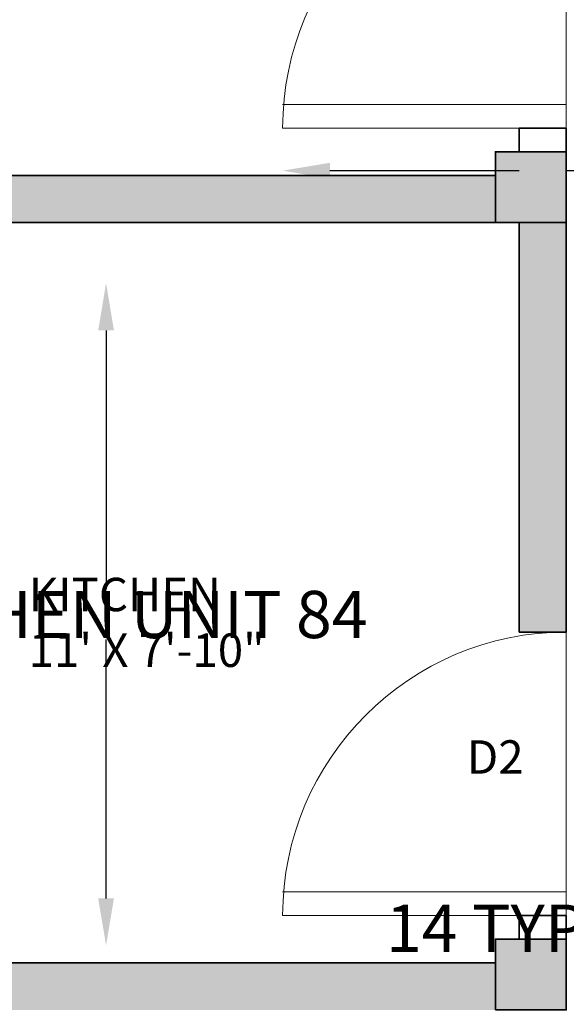
# Model space of a CAD drawing. Units: inches. Extents: x 1994 to 3075, y 3517 to 3950.
# Tile 51 of 58: x 2747 to 2816, y 3656 to 3781. Entities that reach past the tile are written whole.
import ezdxf

# ---------------------------------------------------------------- set-up
doc = ezdxf.new("R2010")
doc.units = ezdxf.units.IN
for name, color, linetype, lineweight in [('A-ANNO-DIMS', 2, 'Continuous', 18), ('A-ANNO-TEXT', 7, 'Continuous', 18), ('A-AREA-IDEN', 7, 'Continuous', 18), ('A-COLS', 7, 'Continuous', 35), ('A-COLS-PATT', 6, 'Continuous', 13), ('A-DOOR', 3, 'Continuous', 18), ('A-WALL', 7, 'Continuous', 35), ('A-WALL-PATT', 252, 'Continuous', 13)]:
    doc.layers.add(name, color=color, linetype=linetype, lineweight=lineweight)
doc.styles.get("Standard").update_dxf_attribs({"font": 'arial.ttf'})
doc.dimstyles.get("Standard").update_dxf_attribs({"dimtxt": 6, "dimasz": 6, "dimexe": 0.18, "dimexo": 0.0625, "dimgap": 0.09, "dimtad": 0, "dimtih": 1, "dimtoh": 1, "dimdec": 4, "dimzin": 0, "dimdsep": 46, "dimlunit": 4, "dimtxsty": 'Standard', "dimcen": 0.09, "dimse1": 1, "dimse2": 1, "dimadec": 0, "dimazin": 0, "dimtfac": 1, "dimtdec": 4, "dimtofl": 0, "dimtmove": 0, "dimatfit": 3, "dimfxl": 1, "dimtolj": 1, "dimtzin": 0, "dimarcsym": 0})

# ---------------------------------------------------------------- blocks, each defined once
blk = doc.blocks.new('DOOR-SWING-36IN')
for p, q in [((36, 0), (36, 36)), ((36, 36), (36, 0)), ((0, 3), (36, 3)), ((36, 0), (0, 0)), ((0, 0), (36, 0))]:
    blk.add_line(p, q)
blk.add_arc((36, 0), 36, 90, 180)
blk = doc.blocks.new('*D16')
at = {"layer": 'A-ANNO-DIMS', "color": 0, "lineweight": -2, "transparency": 16777216}
for p, q in [((2827.4, 3679.62), (2827.4, 3677.51)), ((2827.4, 3671.51), (2827.4, 3665.51)), ((2827.4, 3665.51), (2821.4, 3665.51))]:
    blk.add_line(p, q, dxfattribs=at)
at = {"layer": 'A-ANNO-DIMS', "color": 0, "transparency": 16777216}
for points in [[(2826.4, 3679.62), (2828.4, 3679.62), (2827.4, 3685.62)], [(2826.4, 3677.51), (2828.4, 3677.51), (2827.4, 3671.51)]]:
    blk.add_solid(points, dxfattribs=at)
at = {"layer": 'Defpoints', "color": 0, "transparency": 16777216}
for p in [(2829.85, 3685.62), (2827.4, 3671.51), (2829.85, 3671.51)]:
    blk.add_point(p, dxfattribs=at)
at = {"layer": 'A-ANNO-DIMS', "color": 0, "transparency": 16777216, "insert": (2806.99, 3665.51), "char_height": 6, "attachment_point": 5}
blk.add_mtext('\\A1;14 TYP.', dxfattribs=at)
blk = doc.blocks.new('*D21')
at = {"layer": 'A-ANNO-DIMS', "color": 0, "lineweight": -2, "transparency": 16777216}
for p, q in [((2786.07, 3761.73), (2810.07, 3761.73)), ((2816.07, 3761.73), (2822.07, 3761.73))]:
    blk.add_line(p, q, dxfattribs=at)
at = {"layer": 'A-ANNO-DIMS', "color": 0, "transparency": 16777216}
for points in [[(2786.07, 3762.73), (2786.07, 3760.73), (2780.07, 3761.73)], [(2810.07, 3762.73), (2810.07, 3760.73), (2816.07, 3761.73)]]:
    blk.add_solid(points, dxfattribs=at)
at = {"layer": 'Defpoints', "color": 0, "transparency": 16777216}
for p in [(2780.07, 3767.13), (2816.07, 3767.13), (2816.07, 3761.73)]:
    blk.add_point(p, dxfattribs=at)
at = {"layer": 'A-ANNO-DIMS', "color": 0, "transparency": 16777216, "insert": (2865.85, 3761.73), "char_height": 6, "attachment_point": 5}
blk.add_mtext('\\A1;SWING DOOR 36 TYP.', dxfattribs=at)
blk = doc.blocks.new('*D22')
at = {"layer": 'A-ANNO-DIMS', "color": 0, "lineweight": -2, "transparency": 16777216}
for p, q in [((2821.47, 3797.13), (2821.47, 3788.28)), ((2821.47, 3773.13), (2821.47, 3781.97))]:
    blk.add_line(p, q, dxfattribs=at)
at = {"layer": 'A-ANNO-DIMS', "color": 0, "transparency": 16777216}
for points in [[(2820.47, 3797.13), (2822.47, 3797.13), (2821.47, 3803.13)], [(2820.47, 3773.13), (2822.47, 3773.13), (2821.47, 3767.13)]]:
    blk.add_solid(points, dxfattribs=at)
at = {"layer": 'Defpoints', "color": 0, "transparency": 16777216}
for p in [(2816.07, 3803.13), (2821.47, 3803.13), (2816.07, 3767.13)]:
    blk.add_point(p, dxfattribs=at)
at = {"layer": 'A-ANNO-DIMS', "color": 0, "transparency": 16777216, "insert": (2821.47, 3785.13), "char_height": 6, "attachment_point": 5}
blk.add_mtext('\\A1;36 TYP.', dxfattribs=at)
blk = doc.blocks.new('*D29')
at = {"layer": 'A-ANNO-DIMS', "color": 0, "lineweight": -2, "transparency": 16777216}
for p, q in [((2757.66, 3741.43), (2757.66, 3708.56)), ((2757.66, 3669.3), (2757.66, 3702.17))]:
    blk.add_line(p, q, dxfattribs=at)
at = {"layer": 'A-ANNO-DIMS', "color": 0, "transparency": 16777216}
for points in [[(2756.66, 3741.43), (2758.66, 3741.43), (2757.66, 3747.43)], [(2756.66, 3669.3), (2758.66, 3669.3), (2757.66, 3663.3)]]:
    blk.add_solid(points, dxfattribs=at)
at = {"layer": 'Defpoints', "color": 0, "transparency": 16777216}
for p in [(2745.04, 3747.43), (2757.66, 3747.43), (2745.04, 3663.3)]:
    blk.add_point(p, dxfattribs=at)
at = {"layer": 'A-ANNO-DIMS', "color": 0, "transparency": 16777216, "insert": (2757.66, 3705.36), "char_height": 6, "attachment_point": 5}
blk.add_mtext('\\A1;KITCHEN UNIT 84', dxfattribs=at)
blk = doc.blocks.new('*D32')
at = {"layer": 'A-ANNO-DIMS', "color": 0, "lineweight": -2, "transparency": 16777216}
for p, q in [((2636.61, 3908.13), (2636.61, 3730.78)), ((2636.61, 3547.13), (2636.61, 3724.47))]:
    blk.add_line(p, q, dxfattribs=at)
at = {"layer": 'A-ANNO-DIMS', "color": 0, "transparency": 16777216}
for points in [[(2635.61, 3908.13), (2637.61, 3908.13), (2636.61, 3914.13)], [(2635.61, 3547.13), (2637.61, 3547.13), (2636.61, 3541.13)]]:
    blk.add_solid(points, dxfattribs=at)
at = {"layer": 'Defpoints', "color": 0, "transparency": 16777216}
for p in [(2636.61, 3914.13), (2669.07, 3914.13), (2810.07, 3541.13)]:
    blk.add_point(p, dxfattribs=at)
at = {"layer": 'A-ANNO-DIMS', "color": 0, "transparency": 16777216, "insert": (2636.61, 3727.63), "char_height": 6, "attachment_point": 5}
blk.add_mtext('\\A1;373', dxfattribs=at)

msp = doc.modelspace()

# ---------------------------------------------------------------- hatches: boundary and pattern name
at = {"layer": 'A-COLS-PATT'}
h = msp.add_hatch(color=256, dxfattribs=at)
h.dxf.hatch_style = 1
h.paths.add_polyline_path([(2678.072, 3914.1269), (2669.072, 3914.1269), (2669.072, 3905.1269), (2678.072, 3905.1269)])
h.paths.add_polyline_path([(2816.072, 3914.1269), (2807.072, 3914.1269), (2807.072, 3905.1269), (2816.072, 3905.1269)])
h.paths.add_polyline_path([(2894.9096, 3914.1269), (2885.9096, 3914.1269), (2885.9096, 3905.1269), (2894.9096, 3905.1269)])
h.paths.add_polyline_path([(3033.072, 3914.1269), (3024.072, 3914.1269), (3024.072, 3905.1269), (3033.072, 3905.1269)])
h.paths.add_polyline_path([(3033.072, 3764.1269), (3024.072, 3764.1269), (3024.072, 3755.1269), (3033.072, 3755.1269)])
h.paths.add_polyline_path([(2895.072, 3764.1269), (2886.072, 3764.1269), (2886.072, 3755.1269), (2895.072, 3755.1269)])
h.paths.add_polyline_path([(2816.072, 3764.1269), (2807.072, 3764.1269), (2807.072, 3755.1269), (2816.072, 3755.1269)])
h.paths.add_polyline_path([(2678.072, 3764.1269), (2669.072, 3764.1269), (2669.072, 3755.1269), (2678.072, 3755.1269)])
h.paths.add_polyline_path([(2678.072, 3664.1269), (2669.072, 3664.1269), (2669.072, 3655.1269), (2678.072, 3655.1269)])
h.paths.add_polyline_path([(2816.072, 3664.1269), (2807.072, 3664.1269), (2807.072, 3655.1269), (2816.072, 3655.1269)])
h.paths.add_polyline_path([(3033.072, 3616.1269), (3024.072, 3616.1269), (3024.072, 3607.1269), (3033.072, 3607.1269)])
h.paths.add_polyline_path([(2894.9096, 3616.1269), (2885.9096, 3616.1269), (2885.9096, 3607.1269), (2894.9096, 3607.1269)])
h.paths.add_polyline_path([(2816.072, 3559.1269), (2807.072, 3559.1269), (2807.072, 3550.1269), (2816.072, 3550.1269)])
h.paths.add_polyline_path([(2678.072, 3559.1269), (2669.072, 3559.1269), (2669.072, 3550.1269), (2678.072, 3550.1269)])
at = {"layer": 'A-WALL-PATT'}
h = msp.add_hatch(color=256, dxfattribs=at)
h.dxf.hatch_style = 1
h.paths.add_polyline_path([(2678.072, 3755.1269), (2669.072, 3755.1269), (2669.072, 3718.5523), (2678.072, 3718.5523)])
h.paths.add_polyline_path([(2807.072, 3761.1269), (2678.072, 3761.1269), (2678.072, 3755.1269), (2807.072, 3755.1269)])
h.paths.add_polyline_path([(2678.072, 3812.7371), (2669.072, 3812.7371), (2669.072, 3809.7371), (2669.072, 3764.1269), (2678.072, 3764.1269)])
h.paths.add_polyline_path([(2678.072, 3905.1269), (2669.072, 3905.1269), (2669.072, 3868.7491), (2678.072, 3868.7491)])
h.paths.add_polyline_path([(2723.826, 3914.1269), (2720.826, 3914.1269), (2678.072, 3914.1269), (2678.072, 3905.1269), (2723.826, 3905.1269)])
h.paths.add_polyline_path([(2807.072, 3914.1269), (2779.838, 3914.1269), (2779.838, 3905.1269), (2807.072, 3905.1269)])
h.paths.add_polyline_path([(2837.6979, 3914.1269), (2834.6979, 3914.1269), (2820.9062, 3914.1269), (2816.072, 3914.1269), (2816.072, 3905.1269), (2837.6979, 3905.1269)])
h.paths.add_polyline_path([(2885.9096, 3914.1269), (2869.71, 3914.1269), (2869.71, 3905.1269), (2876.9183, 3905.1269), (2885.9096, 3905.1269)])
h.paths.add_polyline_path([(2933.6904, 3914.1269), (2930.6904, 3914.1269), (2894.9096, 3914.1269), (2894.9096, 3905.1269), (2933.6904, 3905.1269)])
h.paths.add_polyline_path([(3024.072, 3914.1269), (2989.7025, 3914.1269), (2989.7025, 3905.1269), (3024.072, 3905.1269)])
h.paths.add_polyline_path([(3033.072, 3905.1269), (3024.072, 3905.1269), (3024.072, 3861.4192), (3033.072, 3861.4192)])
h.paths.add_polyline_path([(3033.072, 3805.4072), (3024.072, 3805.4072), (3024.072, 3764.1269), (3033.072, 3764.1269)])
h.paths.add_polyline_path([(3033.072, 3755.1269), (3024.072, 3755.1269), (3024.072, 3732.1247), (3033.072, 3732.1247), (3033.072, 3735.1247)])
h.paths.add_polyline_path([(3024.072, 3761.1269), (2895.072, 3761.1269), (2895.072, 3755.1269), (3024.072, 3755.1269)])
h.paths.add_polyline_path([(3033.072, 3676.1126), (3024.072, 3676.1126), (3024.072, 3616.1269), (3033.072, 3616.1269)])
h.paths.add_polyline_path([(3024.072, 3613.1269), (2959.4908, 3613.1269), (2959.4908, 3607.1269), (3024.072, 3607.1269)])
h.paths.add_polyline_path([(2914.1254, 3613.1269), (2894.9096, 3613.1269), (2894.9096, 3607.1269), (2914.1254, 3607.1269)])
h.paths.add_polyline_path([(2885.9096, 3613.1269), (2852.072, 3613.1269), (2852.072, 3607.1269), (2885.9096, 3607.1269)])
h.paths.add_polyline_path([(2822.072, 3613.1269), (2810.072, 3613.1269), (2810.072, 3559.1269), (2816.072, 3559.1269), (2816.072, 3607.1269), (2822.072, 3607.1269)])
h.paths.add_polyline_path([(2933.072, 3607.1269), (2924.072, 3607.1269), (2924.072, 3550.1269), (2892.072, 3550.1269), (2816.072, 3550.1269), (2810.072, 3550.1269), (2810.072, 3541.1269), (2892.072, 3541.1269), (2933.072, 3541.1269)])
h.paths.add_polyline_path([(2807.072, 3559.1269), (2678.072, 3559.1269), (2678.072, 3550.1269), (2807.072, 3550.1269)])
h.paths.add_polyline_path([(2678.072, 3655.1269), (2669.072, 3655.1269), (2669.072, 3559.1269), (2678.072, 3559.1269)])
h.paths.add_polyline_path([(2678.072, 3686.5403), (2669.072, 3686.5403), (2669.072, 3664.1269), (2678.072, 3664.1269)])
h.paths.add_polyline_path([(2807.072, 3661.1269), (2678.072, 3661.1269), (2678.072, 3655.1269), (2807.072, 3655.1269)])
h.paths.add_polyline_path([(2816.072, 3755.1269), (2810.072, 3755.1269), (2810.072, 3703.1269), (2816.072, 3703.1269)])
h.paths.add_polyline_path([(2816.072, 3905.1269), (2810.072, 3905.1269), (2810.072, 3803.1269), (2816.072, 3803.1269), (2816.072, 3815.1269)])
h.paths.add_polyline_path([(2886.072, 3821.1269), (2852.072, 3821.1269), (2852.072, 3815.1269), (2886.072, 3815.1269)])
h.paths.add_polyline_path([(2822.072, 3821.1269), (2816.072, 3821.1269), (2816.072, 3815.1269), (2822.072, 3815.1269)])
h.paths.add_polyline_path([(2892.072, 3905.1269), (2886.072, 3905.1269), (2886.072, 3803.1269), (2892.072, 3803.1269)])

# ---------------------------------------------------------------- linework, layer by layer
at = {"layer": 'A-COLS'}
for points in [[(2807.072, 3755.1269), (2816.072, 3755.1269), (2816.072, 3764.1269), (2807.072, 3764.1269)], [(2807.072, 3655.1269), (2816.072, 3655.1269), (2816.072, 3664.1269), (2807.072, 3664.1269)]]:
    msp.add_lwpolyline(points, close=True, dxfattribs=at)
at = {"layer": 'A-WALL'}
for p, q in [((2810.072, 3764.1269), (2810.072, 3767.1269)), ((2810.072, 3767.1269), (2816.072, 3767.1269)), ((2810.072, 3767.1269), (2810.072, 3764.1269)), ((2816.072, 3767.1269), (2816.072, 3703.1269)), ((2678.072, 3761.1269), (2807.072, 3761.1269)), ((2678.072, 3755.1269), (2810.072, 3755.1269)), ((2810.072, 3755.1269), (2810.072, 3703.1269)), ((2816.072, 3703.1269), (2810.072, 3703.1269)), ((2810.072, 3664.1269), (2810.072, 3667.1269)), ((2810.072, 3667.1269), (2816.072, 3667.1269)), ((2810.072, 3667.1269), (2810.072, 3664.1269)), ((2816.072, 3667.1269), (2816.072, 3661.1269)), ((2816.072, 3667.1269), (2816.072, 3655.1269)), ((2678.072, 3661.1269), (2807.072, 3661.1269))]:
    msp.add_line(p, q, dxfattribs=at)

# ---------------------------------------------------------------- block references
at = {"layer": 'A-DOOR'}
for p in [(2780.072, 3767.127), (2780.072, 3667.127)]:
    msp.add_blockref('DOOR-SWING-36IN', p, dxfattribs=at)

# ---------------------------------------------------------------- texts
at = {"layer": 'A-ANNO-TEXT', "insert": (2803.4532, 3689.3788), "char_height": 4.24528, "attachment_point": 1}
msp.add_mtext_dynamic_manual_height_columns('D2', width=102.693633, gutter_width=21.2264, heights=[0], dxfattribs=at)
at = {"layer": 'A-AREA-IDEN', "insert": (2747.8405, 3710.0212), "char_height": 4.245283, "attachment_point": 1}
msp.add_mtext_dynamic_manual_height_columns('KITCHEN\\P11\' X 7\'-10"', width=102.693633, gutter_width=21.2264, heights=[0], dxfattribs=at)

# ---------------------------------------------------------------- dimensions: what is measured, and where the dimension line sits
at = {"layer": 'A-ANNO-DIMS'}
dim = msp.add_linear_dim(base=(2636.6096, 3914.1269), p1=(2810.072, 3541.1269), p2=(2669.072, 3914.1269), angle=90, dimstyle='Standard', override={"dimdec": 0, "dimlfac": 1, "dimrnd": 0, "dimzin": 0, "dimdsep": 46, "dimlunit": 2}, dxfattribs=at)
dim.commit()
dim.dimension.update_dxf_attribs({"geometry": '*D32', "text_midpoint": (2636.6096, 3727.6269)})
for base, p1, p2, angle, text, picture, middle in [((2821.472, 3803.1269), (2816.072, 3767.1269), (2816.072, 3803.1269), 90, '<> TYP.', '*D22', (2821.472, 3785.1269)), ((2757.6633, 3747.4285), (2745.0442, 3663.3012), (2745.0442, 3747.4285), 90, 'KITCHEN UNIT <>', '*D29', (2757.6633, 3705.3649)), ((2827.4041, 3671.5122), (2829.8543, 3685.6199), (2829.8543, 3671.5122), 270, '<> TYP.', '*D16', (2806.9935, 3665.5122))]:
    dim = msp.add_linear_dim(base=base, p1=p1, p2=p2, angle=angle, text=text, dimstyle='Standard', override={"dimdec": 0, "dimlfac": 1, "dimrnd": 0, "dimzin": 0, "dimdsep": 46, "dimlunit": 2}, dxfattribs=at)
    dim.commit()
    dim.dimension.update_dxf_attribs({"geometry": picture, "text_midpoint": middle})
dim = msp.add_linear_dim(base=(2816.072, 3761.7269), p1=(2780.072, 3767.1269), p2=(2816.072, 3767.1269), text='SWING DOOR <> TYP.', dimstyle='Standard', override={"dimdec": 0, "dimlfac": 1, "dimrnd": 0, "dimzin": 0, "dimdsep": 46, "dimlunit": 2}, dxfattribs=at)
dim.commit()
dim.dimension.update_dxf_attribs({"geometry": '*D21', "text_midpoint": (2865.8544, 3761.7269)})

doc.saveas('drawing.dxf')
